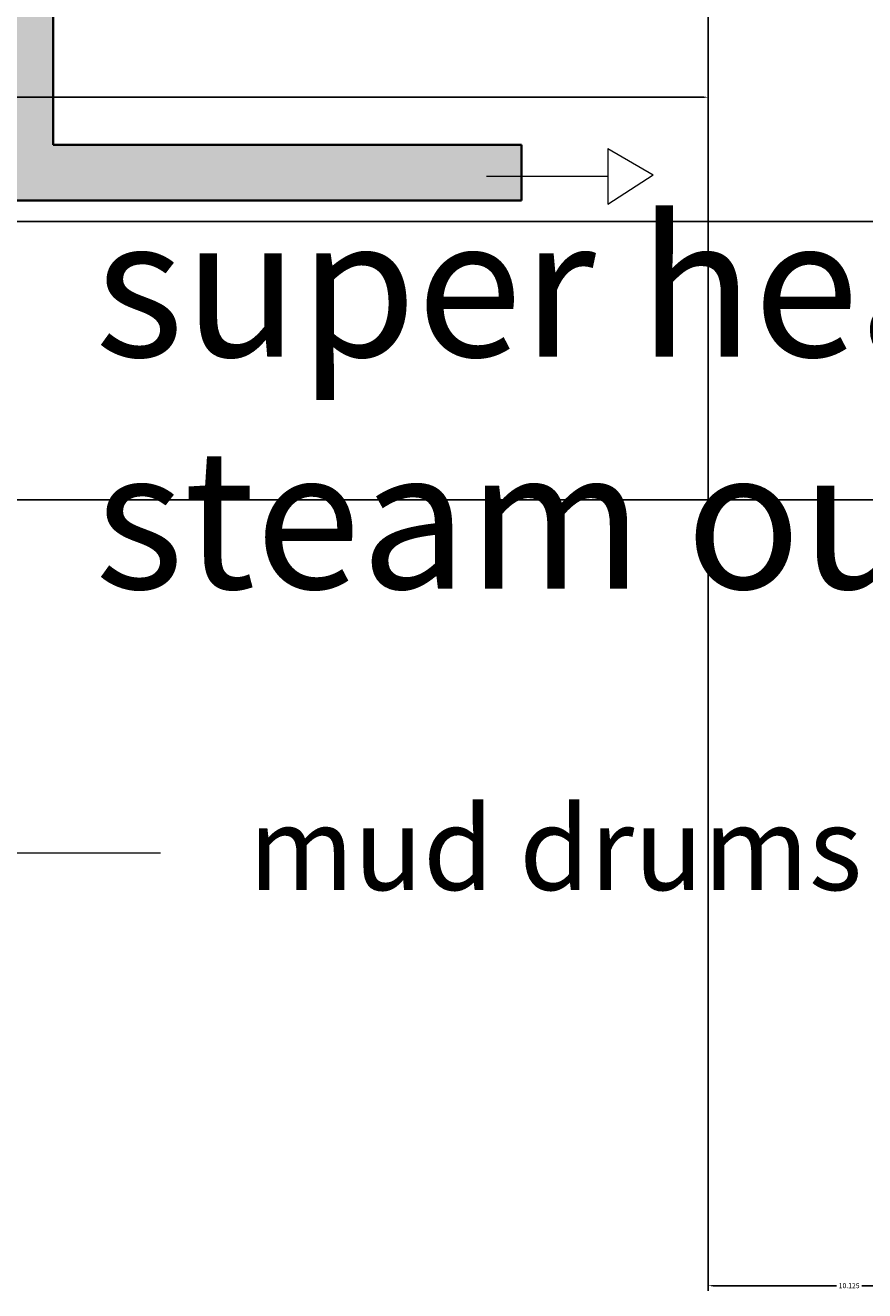
# Model space of a CAD drawing. Units: inches. Extents: x -1 to 292, y -3 to 199.
# Tile 33 of 52: x 181 to 211, y -3 to 43. Entities that reach past the tile are written whole.
import ezdxf

# ---------------------------------------------------------------- set-up
doc = ezdxf.new("R2010")
doc.units = ezdxf.units.IN
doc.header["$MEASUREMENT"] = 0
for name, color, linetype, lineweight in [('M-ANNO-LEAD', 2, 'Continuous', 18), ('M-ANNO-SYMB', 1, 'Continuous', 18), ('M-ANNO-TEXT', 3, 'Continuous', 25), ('M-DIMS', 2, 'Continuous', 18), ('M-EQPM', 7, 'Continuous', 35), ('M-PATT', 8, 'Continuous', 13)]:
    doc.layers.add(name, color=color, linetype=linetype, lineweight=lineweight)
doc.styles.get("Standard").update_dxf_attribs({"font": 'arial.ttf'})
doc.dimstyles.get("Standard").update_dxf_attribs({"dimtxt": 0.18, "dimasz": 0.18, "dimexe": 0.18, "dimexo": 0.0625, "dimgap": 0.09, "dimtad": 0, "dimtih": 1, "dimtoh": 1, "dimdec": 4, "dimzin": 0, "dimdsep": 46, "dimtxsty": 'Standard', "dimcen": 0.09, "dimadec": 0, "dimazin": 0, "dimtfac": 1, "dimtdec": 4, "dimtofl": 0, "dimtmove": 0, "dimatfit": 3, "dimfxl": 1, "dimtolj": 1, "dimtzin": 0, "dimarcsym": 0})

# ---------------------------------------------------------------- blocks, each defined once
blk = doc.blocks.new('FLOW-ARROW-GAS')
for p, q in [((201.507, 38.14), (201.507, 36.14)), ((201.507, 38.14), (203.137, 37.199)), ((201.507, 37.14), (197.151, 37.14)), ((201.507, 36.14), (203.137, 37.199))]:
    blk.add_line(p, q)
blk = doc.blocks.new('*D7')
at = {"layer": 'Defpoints', "color": 0, "transparency": 16777216}
for p in [(21.861, 54.582), (205.115, 54.582), (21.861, 39.982)]:
    blk.add_point(p, dxfattribs=at)
at = {"layer": 'M-DIMS', "color": 0, "lineweight": -2, "transparency": 16777216}
for p, q in [((21.861, 54.52), (21.861, 39.802)), ((205.115, 54.52), (205.115, 39.802)), ((22.041, 39.982), (113.033, 39.982)), ((204.935, 39.982), (113.944, 39.982))]:
    blk.add_line(p, q, dxfattribs=at)
at = {"layer": 'M-DIMS', "color": 0, "transparency": 16777216}
for points in [[(22.041, 40.012), (22.041, 39.952), (21.861, 39.982)], [(204.935, 40.012), (204.935, 39.952), (205.115, 39.982)]]:
    blk.add_solid(points, dxfattribs=at)
at = {"layer": 'M-DIMS', "color": 0, "transparency": 16777216, "insert": (113.488, 39.982), "char_height": 0.18, "attachment_point": 5}
blk.add_mtext('\\A1;183.25', dxfattribs=at)
blk = doc.blocks.new('*D11')
at = {"layer": 'Defpoints', "color": 0, "transparency": 16777216}
for p in [(79.013, 35.514), (292.04, 35.514), (79.013, 25.514)]:
    blk.add_point(p, dxfattribs=at)
at = {"layer": 'M-DIMS', "color": 0, "lineweight": -2, "transparency": 16777216}
for p, q in [((79.076, 35.514), (292.22, 35.514)), ((292.04, 35.334), (292.04, 30.696)), ((292.04, 25.694), (292.04, 30.332)), ((79.076, 25.514), (292.22, 25.514))]:
    blk.add_line(p, q, dxfattribs=at)
at = {"layer": 'M-DIMS', "color": 0, "transparency": 16777216}
for points in [[(292.01, 35.334), (292.07, 35.334), (292.04, 35.514)], [(292.01, 25.694), (292.07, 25.694), (292.04, 25.514)]]:
    blk.add_solid(points, dxfattribs=at)
at = {"layer": 'M-DIMS', "color": 0, "transparency": 16777216, "insert": (292.04, 30.514), "char_height": 0.18, "attachment_point": 5}
blk.add_mtext('\\A1;10', dxfattribs=at)
blk = doc.blocks.new('*D24')
at = {"layer": 'Defpoints', "color": 0, "transparency": 16777216}
for p in [(215.241, 55.034), (205.115, 54.582), (215.241, -2.71)]:
    blk.add_point(p, dxfattribs=at)
at = {"layer": 'M-DIMS', "color": 0, "lineweight": -2, "transparency": 16777216}
for p, q in [((215.241, 54.971), (215.241, -2.89)), ((205.115, 54.52), (205.115, -2.89)), ((205.295, -2.71), (209.722, -2.71)), ((215.061, -2.71), (210.634, -2.71))]:
    blk.add_line(p, q, dxfattribs=at)
at = {"layer": 'M-DIMS', "color": 0, "transparency": 16777216}
for points in [[(205.295, -2.68), (205.295, -2.74), (205.115, -2.71)], [(215.061, -2.68), (215.061, -2.74), (215.241, -2.71)]]:
    blk.add_solid(points, dxfattribs=at)
at = {"layer": 'M-DIMS', "color": 0, "transparency": 16777216, "insert": (210.178, -2.71), "char_height": 0.18, "attachment_point": 5}
blk.add_mtext('\\A1;10.125', dxfattribs=at)

msp = doc.modelspace()

# ---------------------------------------------------------------- hatches: boundary and pattern name
at = {"layer": 'M-PATT'}
h = msp.add_hatch(color=256, dxfattribs=at)
h.set_gradient(color1=(0, 127, 0), color2=(0, 127, 0), tint=1, name='CYLINDER')
h.paths.add_polyline_path([(164.5186, 119.2985), (129.9293, 119.2985), (129.9293, 117.2985), (164.1897, 117.2985)])
h.paths.add_polyline_path([(181.5897, 119.2985), (164.5186, 119.2985), (164.1897, 117.2985), (179.5897, 117.2985), (179.5897, 107.8518), (181.5897, 109.1506)])
h.paths.add_polyline_path([(181.5897, 109.1506), (179.5897, 107.8518), (179.5897, 36.2698), (198.4159, 36.2698), (198.4159, 38.2698), (181.5897, 38.2698)])
h.paths.add_polyline_path([(115.4883, 126.765), (111.4883, 126.765), (111.4883, 114.6589), (115.4883, 114.6589)])
h.paths.add_polyline_path([(123.408, 119.2985), (115.4883, 119.2985), (115.4883, 117.2985), (123.408, 117.2985)])
h.paths.add_polyline_path([(115.4883, 112.6589), (111.4883, 112.6589), (111.4883, 106.9941), (115.4883, 106.9941)])
h.paths.add_polyline_path([(120.9032, 106.9941), (106.0735, 106.9941), (106.0735, 105.9941), (120.9032, 105.9941)])
h.paths.add_polyline_path([(236.4209, 117.5104), (234.9209, 117.5104), (234.9209, 97.1861), (236.4209, 97.1861)])
h.paths.add_polyline_path([(236.4209, 126.4904), (234.9209, 126.4904), (234.9209, 118.9331), (236.4209, 118.9331)])
h.paths.add_polyline_path([(244.9552, 125.7269), (242.9552, 125.7269), (242.9552, 116.8562), (244.9552, 116.8562)])
h.paths.add_polyline_path([(244.9552, 115.1721), (242.9552, 115.1721), (242.9552, 109.7385), (244.9552, 109.7385)])
h.paths.add_polyline_path([(248.4468, 109.7385), (239.4637, 109.7385), (239.4637, 109.4289), (248.4468, 109.4289)])

# ---------------------------------------------------------------- linework, layer by layer
at = {"layer": 'M-ANNO-LEAD'}
msp.add_line((179.3919, 12.8335), (185.4506, 12.8335), dxfattribs=at)
at = {"layer": 'M-EQPM'}
for p, q in [((181.5897, 38.2698), (198.4159, 38.2698)), ((198.4159, 38.2698), (198.4159, 36.2698)), ((179.5897, 36.2698), (198.4159, 36.2698))]:
    msp.add_line(p, q, dxfattribs=at)
msp.add_lwpolyline([(129.9293, 119.2985), (181.5897, 119.2985), (181.5897, 38.2698)], dxfattribs=at)

# ---------------------------------------------------------------- block references
at = {"layer": 'M-ANNO-SYMB'}
msp.add_blockref('FLOW-ARROW-GAS', (0, 0), dxfattribs=at)

# ---------------------------------------------------------------- texts
at = {"layer": 'M-ANNO-TEXT', "attachment_point": 1}
for s, width, insert, char_height in [('super heated steam outlet', 47.899539, (183.0839, 35.6644), 5), ('mud drums', 23.906137, (188.6008, 14.5004), 3)]:
    msp.add_mtext_dynamic_manual_height_columns(s, width=width, gutter_width=1, heights=[0], dxfattribs=dict(at, insert=insert, char_height=char_height))

# ---------------------------------------------------------------- dimensions: what is measured, and where the dimension line sits
at = {"layer": 'M-DIMS'}
dim = msp.add_linear_dim(base=(215.2407, -2.7104), p1=(205.1155, 54.5821), p2=(215.2407, 55.0337), dimstyle='Standard', override={"dimdec": 3, "dimlfac": 1, "dimrnd": 0, "dimzin": 0, "dimdsep": 46, "dimlunit": 2}, dxfattribs=at)
dim.commit()
dim.dimension.update_dxf_attribs({"geometry": '*D24', "text_midpoint": (210.1781, -2.7104)})
for base, p1, p2, angle, override, picture, middle in [((21.8612, 39.9821), (205.1155, 54.5821), (21.8612, 54.5821), 180, {"dimdec": 2, "dimlfac": 1, "dimrnd": 0, "dimzin": 0, "dimdsep": 46, "dimlunit": 2}, '*D7', (113.4883, 39.9821)), ((292.0399, 35.5141), (79.013, 25.5141), (79.013, 35.5141), 90, {"dimdec": 0, "dimlfac": 1, "dimrnd": 0, "dimzin": 0, "dimdsep": 46, "dimlunit": 2}, '*D11', (292.0399, 30.5141))]:
    dim = msp.add_linear_dim(base=base, p1=p1, p2=p2, angle=angle, dimstyle='Standard', override=override, dxfattribs=at)
    dim.commit()
    dim.dimension.update_dxf_attribs({"geometry": picture, "text_midpoint": middle})

doc.saveas('drawing.dxf')
